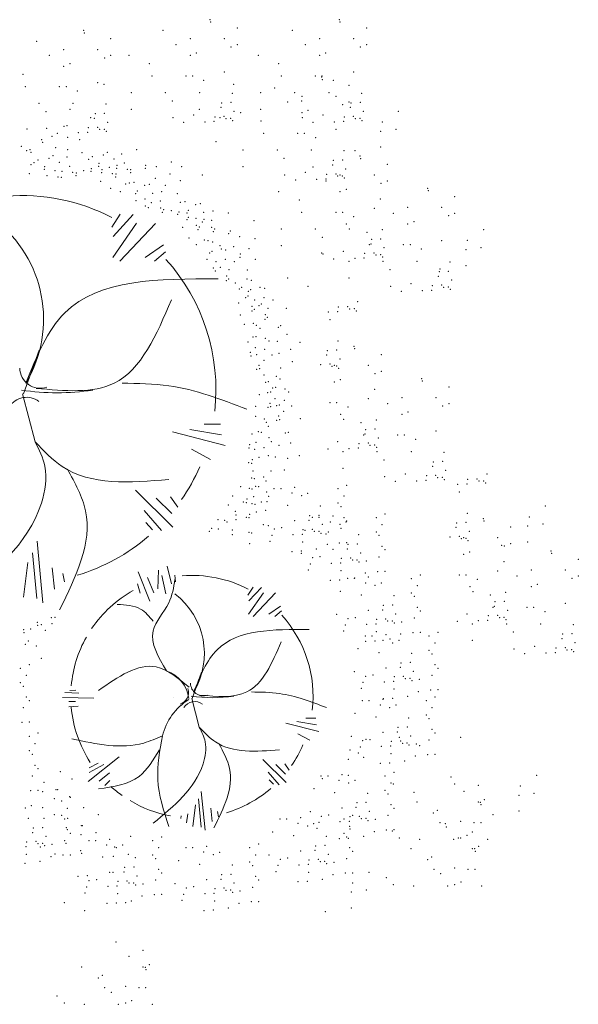
# Model space of a CAD drawing. Units: inches. Extents: x 1239 to 2276906, y 2273 to 321338.
# Tile 21 of 23: x 67989 to 68128, y 11297 to 11541. Entities that reach past the tile are written whole.
import ezdxf

# ---------------------------------------------------------------- set-up
doc = ezdxf.new("R2010")
doc.units = ezdxf.units.IN
doc.layers.add('L-PLNT', color=94, linetype='Continuous', lineweight=13)

# ---------------------------------------------------------------- blocks, each defined once
blk = doc.blocks.new('A$C30B31857')
for p, q in [((3.7503, 4.8792), (3.8028, 4.9604)), ((3.7602, 4.8213), (3.8844, 4.9577)), ((3.7571, 4.688), (3.9054, 4.9034)), ((3.8017, 4.6661), (4.0258, 4.9023)), ((3.9592, 4.6879), (4.0761, 4.7684)), ((4.0192, 4.6658), (4.0886, 4.7234)), ((3.1958, 3.8318), (3.2938, 4.1078)), ((3.1896, 3.8318), (3.2693, 3.5312)), ((4.4619, 3.5087), (4.1316, 3.5937)), ((4.4386, 3.5753), (4.2411, 3.6098)), ((4.4331, 3.6423), (4.3299, 3.6433)), ((4.3707, 3.4211), (4.2509, 3.485)), ((4.1343, 2.9958), (3.8994, 3.2279)), ((4.1284, 3.0819), (4.0285, 3.1775)), ((4.1656, 3.1221), (4.1189, 3.1852)), ((4.0628, 2.975), (3.9547, 3.1008)), ((4.0069, 2.9798), (3.9644, 3.0251)), ((3.3185, 2.5196), (3.2812, 2.9071)), ((3.2801, 2.5477), (3.2528, 2.8343)), ((3.196, 2.5571), (3.224, 2.7743)), ((3.39, 2.6068), (3.3766, 2.7403)), ((4.0388, 2.6092), (4.0438, 2.7263)), ((4.1263, 2.6395), (4.0978, 2.7511)), ((3.4532, 2.6516), (3.4426, 2.7052)), ((3.9897, 2.5318), (3.9158, 2.7153)), ((4.0155, 2.5826), (3.975, 2.6798)), ((4.0896, 2.578), (4.065, 2.6912)), ((4.1506, 2.6527), (4.1457, 2.6942)), ((3.928, 2.5823), (3.9112, 2.6389)), ((4.6056, 2.5687), (4.6384, 2.6195)), ((4.6118, 2.5325), (4.6895, 2.6178)), ((4.6098, 2.4492), (4.7026, 2.5839)), ((4.6377, 2.4355), (4.7778, 2.5831)), ((4.7362, 2.4491), (4.8093, 2.4995)), ((4.7737, 2.4353), (4.8171, 2.4714)), ((4.256, 1.9202), (4.3148, 2.0859)), ((3.4418, 1.9254), (3.6381, 1.9223)), ((3.4556, 1.9575), (3.5427, 1.954)), ((3.488, 1.9706), (3.5256, 1.9718)), ((4.2523, 1.9202), (4.3001, 1.7399)), ((3.4801, 1.8674), (3.5393, 1.8722)), ((3.4804, 1.9008), (3.5234, 1.9004)), ((5.0324, 1.7957), (4.9679, 1.7963)), ((5.0504, 1.7122), (4.8439, 1.7653)), ((5.0358, 1.7538), (4.9124, 1.7754)), ((4.9934, 1.6574), (4.9185, 1.6973)), ((3.6033, 1.3996), (3.7969, 1.5536)), ((3.608, 1.4856), (3.6648, 1.5146)), ((3.6093, 1.4548), (3.7012, 1.505)), ((4.8456, 1.3916), (4.6988, 1.5367)), ((4.8419, 1.4454), (4.7795, 1.5052)), ((4.8652, 1.4705), (4.836, 1.51)), ((3.6717, 1.4005), (3.7356, 1.4536)), ((4.8009, 1.3786), (4.7333, 1.4572)), ((3.7064, 1.3744), (3.739, 1.4052)), ((4.766, 1.3816), (4.7394, 1.4099)), ((4.3358, 1.094), (4.3124, 1.3362)), ((4.2592, 1.1174), (4.2766, 1.2532)), ((4.3117, 1.1115), (4.2947, 1.2906)), ((4.1844, 1.1665), (4.1872, 1.1826)), ((4.2206, 1.1393), (4.2277, 1.1957)), ((4.3805, 1.1485), (4.3721, 1.2319)), ((4.4199, 1.1765), (4.4133, 1.21))]:
    blk.add_line(p, q)
for centre, radius, start, end in [((3.1873, 3.861), 1.217, 62.40199, 94.67087), ((2.5377, 4.3028), 0.7844, 329.07822, 52.6009), ((3.1873, 3.861), 1.217, 353.50541, 42.09121), ((3.3005, 3.9951), 0.1272, 180.26687, 289.21544), ((3.4071, 5.3392), 1.4997, 261.42775, 278.57225), ((3.2157, 3.6838), 0.1272, 52.7337, 148.31892), ((3.1873, 3.861), 1.217, 325.31812, 336.41917), ((3.1873, 3.861), 1.217, 286.50052, 310.70203), ((4.2538, 1.9324), 0.7606, 62.40199, 94.67087), ((4.2538, 1.9324), 0.7606, 118.93501, 145.86797), ((3.8611, 2.2029), 0.4706, 329.07822, 52.6009), ((4.2538, 1.9324), 0.7606, 353.50541, 42.09121), ((4.2538, 1.9324), 0.7606, 150.59537, 174.9599), ((4.0258, 1.8951), 0.2096, 6.88406, 70.93506), ((4.153, 1.9587), 0.0795, 289.21544, 17.13172), ((4.3245, 2.0162), 0.0795, 180.26687, 289.21544), ((4.2203, 1.9258), 0.0795, 179.43656, 180.26687), ((4.3827, 2.8247), 0.8998, 261.42775, 278.57225), ((4.2538, 1.9324), 0.7606, 185.11549, 212.96103), ((4.4263, 1.5995), 0.3678, 121.54331, 166.60172), ((4.2715, 1.8216), 0.0795, 52.7337, 148.31892), ((4.2538, 1.9324), 0.7606, 325.31812, 336.41917), ((4.2538, 1.9324), 0.7606, 227.99389, 234.92066), ((4.2538, 1.9324), 0.7606, 286.50052, 310.70203), ((4.2538, 1.9324), 0.7606, 239.25491, 259.86097)]:
    blk.add_arc(centre, radius, start, end)
for points, knots in [([(3.2106, 3.8997), (3.2782, 4.0657), (3.478, 4.5561), (4.0445, 4.5549), (4.4191, 4.5541)], [0, 0, 0, 0, 0.505063, 1.491803, 1.491803, 1.491803, 1.491803]), ([(3.2759, 3.867), (3.4546, 3.8509), (3.8645, 3.8139), (4.0311, 4.2035), (4.1251, 4.4232)], [0, 0, 0, 0, 0.49103, 1.125938, 1.125938, 1.125938, 1.125938]), ([(3.8148, 3.8997), (3.9136, 3.8984), (4.1838, 3.8949), (4.4376, 3.7978), (4.5987, 3.7361)], [0, 0, 0, 0, 0.29442, 0.8060024, 0.8060024, 0.8060024, 0.8060024]), ([(3.2693, 3.5312), (3.2945, 3.4812), (3.355, 3.361), (3.2868, 2.9371), (3.0051, 2.7057), (2.786, 2.5256)], [0, 0, 0, 0, 0.165135, 0.396758, 1.208872, 1.208872, 1.208872, 1.208872]), ([(3.2693, 3.5312), (3.3234, 3.4742), (3.5366, 3.2499), (3.8644, 3.2754), (4.1088, 3.2945)], [0, 0, 0, 0, 0.229976, 0.9045396, 0.9045396, 0.9045396, 0.9045396]), ([(3.4719, 3.3599), (3.5196, 3.2734), (3.6746, 2.9922), (3.5259, 2.6875), (3.4229, 2.4766)], [0, 0, 0, 0, 0.2856103, 0.9283265, 0.9283265, 0.9283265, 0.9283265]), ([(4.0943, 2.0932), (4.0431, 2.1794), (3.9528, 2.3314), (4.1194, 2.5003), (4.1389, 2.6174), (4.1473, 2.6677)], [0, 0, 0, 0, 0.2643394, 0.4663641, 0.6187177, 0.6187177, 0.6187177, 0.6187177]), ([(4.0102, 2.4054), (3.986, 2.4345), (3.9287, 2.5035), (3.8375, 2.508), (3.7847, 2.5106)], [0, 0, 0, 0, 0.1091589, 0.2590609, 0.2590609, 0.2590609, 0.2590609]), ([(4.2649, 1.961), (4.3054, 2.0606), (4.4253, 2.3548), (4.7652, 2.3541), (4.99, 2.3536)], [0, 0, 0, 0, 0.303038, 0.8950819, 0.8950819, 0.8950819, 0.8950819]), ([(4.3041, 1.9414), (4.4113, 1.9317), (4.6572, 1.9095), (4.7572, 2.1433), (4.8136, 2.2751)], [0, 0, 0, 0, 0.2946182, 0.675563, 0.675563, 0.675563, 0.675563]), ([(4.2355, 1.9904), (4.1681, 2.0469), (3.9917, 2.1946), (3.7911, 2.0563), (3.6671, 1.9708)], [0, 0, 0, 0, 0.2421239, 0.6334325, 0.6334325, 0.6334325, 0.6334325]), ([(4.6274, 1.961), (4.6866, 1.9602), (4.8488, 1.9581), (5.0011, 1.8998), (5.0978, 1.8629)], [0, 0, 0, 0, 0.176652, 0.4836014, 0.4836014, 0.4836014, 0.4836014]), ([(4.3001, 1.7399), (4.3152, 1.7099), (4.3515, 1.6377), (4.3106, 1.3834), (4.1416, 1.2446), (4.0101, 1.1365)], [0, 0, 0, 0, 0.0990809, 0.2380551, 0.7253232, 0.7253232, 0.7253232, 0.7253232]), ([(4.3001, 1.7399), (4.3326, 1.7057), (4.4604, 1.5711), (4.6571, 1.5864), (4.8038, 1.5978)], [0, 0, 0, 0, 0.1379856, 0.5427238, 0.5427238, 0.5427238, 0.5427238]), ([(4.0689, 1.6862), (4.0299, 1.669), (3.8517, 1.5906), (3.6546, 1.6333), (3.5005, 1.6666)], [0, 0, 0, 0, 0.1264411, 0.5776247, 0.5776247, 0.5776247, 0.5776247]), ([(4.0689, 1.6862), (4.0518, 1.5941), (4.0159, 1.4014), (4.0764, 1.2145), (4.1081, 1.1169)], [0, 0, 0, 0, 0.2763889, 0.5787232, 0.5787232, 0.5787232, 0.5787232]), ([(4.4216, 1.6371), (4.4503, 1.5852), (4.5433, 1.4165), (4.454, 1.2337), (4.3922, 1.1071)], [0, 0, 0, 0, 0.1713662, 0.5569959, 0.5569959, 0.5569959, 0.5569959]), ([(4.0493, 1.5978), (4.0122, 1.5345), (3.928, 1.3908), (3.7607, 1.3662), (3.6671, 1.3525)], [0, 0, 0, 0, 0.2099222, 0.4765171, 0.4765171, 0.4765171, 0.4765171])]:
    blk.add_open_spline(points, degree=3, knots=knots)
for p in [(4.3671, 6.1817), (5.1793, 6.1817), (4.3711, 6.1664), (4.5382, 6.1295), (5.1833, 6.1664), (5.3504, 6.1295), (3.5734, 6.1141), (3.5774, 6.0988), (3.7445, 6.0619), (4.0717, 6.1142), (4.2428, 6.062), (4.4567, 6.062), (4.8839, 6.1142), (5.055, 6.062), (5.2689, 6.062), (3.278, 6.0466), (4.1532, 6.025), (4.4994, 6.0098), (4.5382, 6.025), (4.9654, 6.025), (5.3116, 6.0098), (5.3504, 6.025), (3.3595, 5.9574), (3.4491, 5.9944), (3.6629, 5.9944), (3.7057, 5.9422), (3.7445, 5.9574), (3.8578, 5.9575), (4.2428, 5.9575), (4.2816, 5.9728), (4.67, 5.9575), (5.055, 5.9575), (5.0937, 5.9728), (3.4491, 5.8899), (3.4878, 5.9052), (3.9861, 5.9053), (4.7983, 5.9053), (3.1924, 5.8377), (4.002, 5.8283), (4.2159, 5.8283), (4.2586, 5.8283), (4.4567, 5.8531), (4.8142, 5.8283), (5.0281, 5.8283), (5.0685, 5.8211), (5.0708, 5.8283), (5.2689, 5.8531), (3.2083, 5.7607), (3.4221, 5.7607), (3.4649, 5.7607), (3.6629, 5.7855), (3.7026, 5.7761), (4.3283, 5.8008), (4.5148, 5.7761), (4.7731, 5.7537), (5.0726, 5.8059), (5.1405, 5.8008), (5.2396, 5.7689), (3.5346, 5.7332), (3.8737, 5.7238), (4.0876, 5.7238), (4.3014, 5.7238), (4.507, 5.7196), (4.6859, 5.7238), (4.8997, 5.7238), (4.9442, 5.7014), (5.1136, 5.7238), (5.1581, 5.7014), (5.3192, 5.7196), (3.2938, 5.6562), (3.5077, 5.6562), (3.7133, 5.652), (4.1303, 5.6716), (4.4356, 5.6305), (4.44, 5.6593), (4.4982, 5.662), (4.8547, 5.6645), (4.9425, 5.6716), (5.2009, 5.6492), (5.2396, 5.6645), (5.2478, 5.6305), (5.2522, 5.6593), (5.3104, 5.662), (3.3366, 5.604), (3.4887, 5.6194), (3.617, 5.5672), (3.6463, 5.5917), (3.7045, 5.5944), (3.8737, 5.6194), (4.1351, 5.5664), (4.2638, 5.5831), (4.3009, 5.6194), (4.3977, 5.5715), (4.4292, 5.5672), (4.4559, 5.5742), (4.5185, 5.6058), (4.5593, 5.597), (4.6859, 5.6194), (4.9442, 5.597), (4.9473, 5.5664), (4.983, 5.6122), (5.076, 5.5831), (5.2099, 5.5715), (5.2681, 5.5742), (5.3307, 5.6058), (5.5495, 5.607), (3.4498, 5.5125), (3.4701, 5.5155), (3.604, 5.5039), (3.6419, 5.5629), (3.6622, 5.5066), (3.7248, 5.5382), (4.2026, 5.5364), (4.3351, 5.54), (4.3933, 5.5427), (4.4683, 5.5605), (4.4974, 5.5619), (4.5097, 5.5482), (4.6876, 5.5447), (5.0148, 5.5364), (5.1473, 5.54), (5.2055, 5.5427), (5.2804, 5.5605), (5.3095, 5.5619), (5.3219, 5.5482), (5.4484, 5.5393), (3.2183, 5.4955), (3.3414, 5.4988), (3.3754, 5.4495), (3.4088, 5.4688), (3.4726, 5.4423), (3.5414, 5.4724), (3.5996, 5.4751), (3.6745, 5.4929), (3.7036, 5.4943), (3.716, 5.4806), (4.7034, 5.4677), (4.9173, 5.4677), (4.9601, 5.4677), (5.0298, 5.4403), (5.1581, 5.4925), (5.4396, 5.4817), (5.5341, 5.4943), (3.1825, 5.3868), (3.3111, 5.4286), (3.3168, 5.4111), (3.3983, 5.3793), (3.5483, 5.4281), (4.404, 5.4155), (5.4388, 5.3816), (3.2153, 5.3587), (3.2368, 5.3657), (3.2368, 5.3657), (3.2425, 5.3481), (3.3807, 5.3283), (3.4704, 5.3189), (3.474, 5.3651), (3.5639, 5.3462), (3.6293, 5.3208), (3.6985, 5.3321), (3.7228, 5.3481), (3.8125, 5.3386), (3.906, 5.3659), (4.5751, 5.3633), (4.789, 5.3633), (5.0029, 5.3633), (5.2085, 5.359), (5.2765, 5.3597), (5.3085, 5.3254), (3.2439, 5.2709), (3.2628, 5.2851), (3.2872, 5.3011), (3.3282, 5.2596), (3.3564, 5.3123), (3.4217, 5.2869), (3.487, 5.2615), (3.6049, 5.3048), (3.6683, 5.261), (3.6703, 5.2794), (3.7638, 5.3066), (3.7823, 5.2676), (3.8291, 5.2812), (3.9636, 5.2671), (4.0309, 5.26), (4.1244, 5.2873), (4.1902, 5.2588), (4.5751, 5.2588), (4.8318, 5.3111), (5.0131, 5.2579), (5.137, 5.2699), (5.1414, 5.2987), (5.1997, 5.3014), (5.3125, 5.3101), (5.4796, 5.2732), (3.2327, 5.214), (3.3262, 5.2413), (3.3448, 5.2022), (3.3935, 5.2342), (3.4121, 5.1951), (3.4345, 5.1928), (3.4383, 5.2295), (3.5056, 5.2224), (3.5261, 5.2017), (3.528, 5.2201), (3.528, 5.2201), (3.5748, 5.2337), (3.6196, 5.229), (3.6216, 5.2474), (3.6869, 5.2219), (3.6888, 5.2403), (3.7356, 5.2539), (3.7541, 5.2149), (3.7746, 5.1942), (3.7766, 5.2125), (3.7804, 5.2492), (3.8477, 5.2421), (3.8682, 5.2214), (3.8701, 5.2398), (3.8701, 5.2398), (3.9617, 5.2487), (4.1167, 5.2139), (4.3185, 5.2066), (4.8366, 5.2059), (4.9652, 5.2226), (5.0991, 5.2109), (5.1573, 5.2137), (5.1697, 5.2), (5.1842, 5.2057), (5.1988, 5.2013), (5.2199, 5.2452), (5.3981, 5.2057), (3.6811, 5.1669), (3.838, 5.1504), (3.8611, 5.1556), (3.8899, 5.1603), (3.9577, 5.1424), (3.9864, 5.1471), (4.0232, 5.1866), (4.0866, 5.1428), (4.1801, 5.1701), (4.904, 5.1758), (5.0365, 5.1794), (5.0946, 5.1687), (5.0947, 5.1821), (5.2111, 5.1876), (5.4408, 5.1534), (5.4796, 5.1687), (3.7445, 5.1231), (3.8047, 5.1029), (3.9012, 5.0898), (3.9105, 5.1058), (4.007, 5.0926), (4.0645, 5.1021), (4.1611, 5.0889), (4.7992, 5.1012), (5.1842, 5.1012), (5.223, 5.1165), (5.7331, 5.1226), (5.7371, 5.1073), (5.9042, 5.0703), (3.9023, 5.0465), (3.9598, 5.056), (3.9609, 5.0127), (3.9989, 5.0334), (4.0564, 5.0428), (4.1817, 5.0344), (4.2104, 5.0391), (4.2782, 5.0213), (4.3069, 5.026), (4.9275, 5.049), (5.4376, 5.0551), (3.9804, 5.0015), (4.0574, 4.9996), (4.0677, 4.9724), (4.0769, 4.9883), (4.0769, 4.9883), (4.1252, 4.9818), (4.1643, 4.9592), (4.1735, 4.9752), (4.2218, 4.9687), (4.231, 4.9846), (4.3275, 4.9715), (4.385, 4.9809), (4.4816, 4.9678), (4.9434, 4.972), (5.1573, 4.972), (5.2, 4.972), (5.3981, 4.9967), (5.5192, 4.9659), (5.6087, 5.0028), (5.8226, 5.0028), (5.8654, 4.9506), (5.9042, 4.9659), (4.2228, 4.9254), (4.2321, 4.9414), (4.2803, 4.9348), (4.2814, 4.8916), (4.3194, 4.9123), (4.3286, 4.9283), (4.3769, 4.9217), (4.644, 4.9198), (5.2238, 4.8984), (5.2697, 4.9445), (5.6087, 4.8984), (5.6475, 4.9136), (4.1951, 4.8775), (4.2917, 4.8644), (4.3009, 4.8803), (4.3779, 4.8785), (4.3882, 4.8512), (4.3975, 4.8672), (4.3975, 4.8672), (4.4848, 4.8381), (4.494, 4.8541), (4.8151, 4.8675), (5.029, 4.8675), (5.2428, 4.8675), (5.3521, 4.8462), (5.4484, 4.8633), (6.0848, 4.8633), (4.2353, 4.8117), (4.282, 4.7688), (4.3318, 4.7986), (4.355, 4.7939), (4.3832, 4.7865), (4.4301, 4.7631), (4.5526, 4.8203), (4.6491, 4.8072), (4.8151, 4.7631), (5.0717, 4.8153), (5.368, 4.7692), (5.377, 4.7741), (5.3814, 4.8029), (5.4396, 4.8057), (5.5818, 4.7692), (5.6246, 4.7692), (5.8226, 4.7939), (5.9837, 4.7957), (4.3649, 4.7175), (4.3798, 4.7283), (4.4379, 4.7427), (4.4661, 4.7353), (4.5157, 4.7564), (4.5584, 4.7108), (4.6122, 4.7432), (5.0685, 4.7169), (5.0765, 4.7101), (5.2052, 4.7268), (5.3391, 4.7152), (5.3973, 4.7179), (5.4097, 4.7042), (5.4388, 4.7056), (5.4599, 4.7495), (5.6943, 4.7417), (5.9749, 4.7381), (6.0694, 4.7506), (4.3483, 4.6776), (4.4047, 4.6628), (4.4627, 4.6771), (4.5191, 4.6623), (4.5558, 4.6906), (4.6523, 4.6775), (5.144, 4.6801), (5.2396, 4.6647), (5.2765, 4.6836), (5.3347, 4.6864), (5.4511, 4.6919), (5.4535, 4.6647), (5.6674, 4.6647), (5.873, 4.6605), (5.9741, 4.638), (4.388, 4.6229), (4.4013, 4.6046), (4.4312, 4.6263), (4.4875, 4.6115), (4.6019, 4.6111), (5.4963, 4.6125), (5.806, 4.6001), (5.8118, 4.616), (5.8642, 4.6029), (4.4692, 4.5425), (4.4709, 4.5716), (4.4842, 4.5534), (4.4842, 4.5534), (4.5256, 4.5277), (4.5986, 4.5529), (4.6267, 4.5455), (4.8547, 4.5603), (5.2396, 4.5603), (5.6298, 4.524), (5.8016, 4.5713), (5.8219, 4.5151), (5.8845, 4.5466), (4.5521, 4.4913), (4.567, 4.5021), (4.6085, 4.4765), (4.6234, 4.4873), (4.6814, 4.5016), (4.7096, 4.4942), (4.983, 4.508), (5.5011, 4.5073), (5.5685, 4.4772), (5.701, 4.4808), (5.7593, 4.4836), (5.7637, 4.5124), (5.8342, 4.5014), (5.8633, 4.5028), (5.8757, 4.489), (4.547, 4.404), (4.5918, 4.4366), (4.6068, 4.4474), (4.6482, 4.4218), (4.6896, 4.3961), (4.7062, 4.4361), (4.7626, 4.4213), (5.2938, 4.4114), (4.5569, 4.3276), (4.6299, 4.3528), (4.6316, 4.3818), (4.6448, 4.3636), (4.6747, 4.3853), (4.7145, 4.3306), (4.7311, 4.3705), (4.8455, 4.37), (5.1104, 4.3456), (5.1686, 4.3484), (5.173, 4.3772), (5.2312, 4.3799), (5.2435, 4.3662), (5.2726, 4.3675), (5.285, 4.3538), (4.5822, 4.2693), (4.6398, 4.2763), (4.7128, 4.3015), (4.7277, 4.3123), (4.7277, 4.3123), (5.1212, 4.2982), (4.6591, 4.2626), (4.6818, 4.2444), (4.7956, 4.2502), (4.8106, 4.2611), (4.8503, 4.2064), (4.6056, 4.1591), (4.6371, 4.1888), (4.6551, 4.1927), (4.714, 4.1821), (4.7367, 4.1639), (4.7906, 4.163), (4.9332, 4.1551), (5.1715, 4.1647), (4.6197, 4.0929), (4.6511, 4.1227), (4.71, 4.1121), (4.8005, 4.0866), (4.8735, 4.1117), (5.1045, 4.1044), (5.1627, 4.1071), (5.2716, 4.131), (5.2756, 4.1158), (4.6244, 4.0709), (4.6605, 4.0786), (4.706, 4.0421), (4.7554, 4.0757), (4.8833, 4.0353), (5.1001, 4.0756), (5.1204, 4.0193), (5.183, 4.0509), (5.4427, 4.0788), (4.6612, 3.9865), (4.6746, 4.0124), (4.6792, 3.9904), (4.6792, 3.9904), (4.8103, 3.9952), (5.0622, 4.0166), (5.1328, 4.0056), (5.1473, 4.0113), (5.1619, 4.007), (5.1742, 3.9933), (5.3611, 4.0113), (5.4039, 3.9591), (5.4427, 3.9743), (4.7067, 3.9501), (4.716, 3.906), (4.7341, 3.9098), (4.7836, 3.9434), (4.8063, 3.9252), (5.1473, 3.9069), (5.186, 3.9221), (5.6961, 3.9282), (5.7001, 3.913), (4.7301, 3.8399), (4.7482, 3.8437), (4.7615, 3.8696), (4.7796, 3.8734), (4.8384, 3.8629), (4.8612, 3.8447), (5.4007, 3.8607), (5.8672, 3.876), (4.6759, 3.8283), (4.7442, 3.7737), (4.7756, 3.8034), (4.8344, 3.7929), (5.1204, 3.7776), (5.1631, 3.7776), (5.3611, 3.8024), (5.4823, 3.7715), (5.5718, 3.8085), (5.7857, 3.8085), (5.8672, 3.7715), (4.6539, 3.7545), (4.7308, 3.7478), (4.7489, 3.7517), (4.785, 3.7593), (4.803, 3.7632), (4.8304, 3.7229), (4.8799, 3.7565), (5.2328, 3.7502), (5.6106, 3.7193), (5.8285, 3.7563), (4.6533, 3.691), (4.7088, 3.674), (4.7208, 3.6536), (4.7857, 3.6673), (4.799, 3.6932), (4.8037, 3.6711), (4.8037, 3.6711), (4.9348, 3.6759), (5.1869, 3.704), (5.2059, 3.6732), (5.3152, 3.6518), (5.4115, 3.6689), (5.5718, 3.704), (4.6707, 3.5951), (4.6887, 3.5913), (4.7342, 3.6277), (4.8405, 3.5868), (4.8586, 3.5906), (5.3445, 3.6086), (5.4027, 3.6113), (5.7857, 3.5996), (4.6299, 3.5808), (4.6566, 3.529), (4.7382, 3.5578), (4.7515, 3.5319), (4.8726, 3.5245), (5.1683, 3.5325), (5.331, 3.5748), (5.3401, 3.5798), (5.423, 3.5551), (5.5449, 3.5748), (5.5877, 3.5748), (5.6574, 3.5474), (4.6111, 3.4926), (4.6158, 3.5146), (4.6472, 3.4849), (4.7061, 3.4954), (4.8004, 3.5091), (5.1071, 3.4857), (5.2027, 3.4704), (5.2396, 3.4893), (5.2978, 3.492), (5.3022, 3.5208), (5.3604, 3.5236), (5.3727, 3.5099), (5.4018, 3.5112), (5.4142, 3.4975), (5.4166, 3.4704), (5.6305, 3.4704), (5.8361, 3.4661), (4.6104, 3.4005), (4.6332, 3.4187), (4.674, 3.4331), (4.7328, 3.4437), (4.7784, 3.4353), (4.8553, 3.4286), (4.9275, 3.4439), (5.4594, 3.4181), (5.769, 3.4058), (5.8273, 3.4085), (4.6285, 3.3967), (4.6285, 3.3967), (4.6372, 3.3488), (4.7502, 3.3478), (4.8332, 3.3548), (5.2027, 3.3659), (5.7646, 3.377), (5.8475, 3.3523), (4.6278, 3.3047), (4.6458, 3.3008), (4.7047, 3.3114), (4.718, 3.2855), (5.4642, 3.3129), (5.5316, 3.2829), (5.5928, 3.3297), (5.6641, 3.2865), (5.7223, 3.2892), (5.7267, 3.318), (5.7849, 3.3208), (5.7973, 3.307), (5.8264, 3.3084), (5.8387, 3.2947), (5.9852, 3.2955), (6.0434, 3.2982), (6.0557, 3.2845), (6.0848, 3.2859), (6.106, 3.3298), (4.5596, 3.25), (4.6137, 3.2385), (4.6318, 3.2347), (4.6545, 3.2529), (4.6726, 3.2491), (4.722, 3.2155), (4.7696, 3.2368), (4.8124, 3.2368), (4.8997, 3.2451), (5.1707, 3.2366), (5.2261, 3.2591), (5.9226, 3.2639), (5.9334, 3.2165), (5.9808, 3.2667), (6.0972, 3.2722), (4.5094, 3.1915), (4.5769, 3.1541), (4.5997, 3.1724), (4.6404, 3.1867), (4.6899, 3.1532), (4.7246, 3.1559), (4.7354, 3.1896), (4.8821, 3.2093), (4.9424, 3.1929), (4.9812, 3.2082), (5.2076, 3.1915), (4.483, 3.1338), (4.5268, 3.0957), (4.595, 3.1503), (4.6311, 3.1426), (4.6491, 3.1388), (4.6578, 3.0909), (4.7167, 3.1014), (4.8552, 3.1323), (5.0608, 3.1281), (5.1707, 3.1464), (5.1892, 3.1239), (6.4724, 3.1281), (4.4168, 3.0426), (4.4599, 3.0391), (4.5295, 3.0722), (4.5312, 3.0431), (4.5943, 3.0583), (4.6123, 3.0544), (4.6123, 3.0544), (4.617, 3.0765), (4.8997, 3.0362), (4.9894, 3.039), (4.9938, 3.0678), (5.0096, 3.0565), (5.052, 3.0705), (5.0524, 3.0565), (5.1221, 3.0291), (5.1396, 3.0649), (5.2076, 3.0562), (5.2261, 3.0337), (5.4107, 3.0563), (5.4661, 3.0788), (5.9837, 3.083), (6.0838, 3.0494), (6.0878, 3.0341), (6.3714, 3.0605), (4.3638, 2.9696), (4.377, 2.9879), (4.4201, 2.9844), (4.4748, 3.0283), (4.5064, 2.9775), (4.7017, 3.0115), (4.734, 3.0055), (4.7714, 2.984), (4.8176, 2.9916), (4.9515, 2.98), (4.9645, 2.9757), (5.0097, 2.9827), (5.022, 2.969), (5.0511, 2.9704), (5.0723, 3.0143), (5.1824, 3.0126), (5.1892, 2.9886), (5.2212, 3.0279), (5.4476, 3.0112), (5.9123, 2.9939), (5.9167, 3.0227), (5.9749, 3.0254), (5.9952, 2.9692), (6.2549, 2.9971), (6.3626, 3.0029), (6.4571, 3.0154), (4.508, 2.9484), (4.6116, 2.9624), (4.6297, 2.9586), (4.7444, 2.907), (4.7563, 2.9449), (4.8889, 2.9485), (4.9471, 2.9512), (5.0635, 2.9567), (5.0952, 2.9521), (5.1094, 2.9645), (5.3008, 2.9478), (5.4107, 2.9661), (5.4292, 2.9436), (5.8744, 2.9349), (5.9326, 2.9377), (5.945, 2.9239), (5.9595, 2.9296), (5.9741, 2.9253), (5.9864, 2.9116), (6.1733, 2.9296), (4.6156, 2.8924), (4.9412, 2.8452), (4.95, 2.9027), (5.0357, 2.8577), (5.1032, 2.8877), (5.1396, 2.8559), (5.1798, 2.8972), (5.2261, 2.8984), (5.2293, 2.8587), (5.2337, 2.8875), (5.2919, 2.8902), (5.4476, 2.8759), (5.4661, 2.8534), (6.1994, 2.8809), (6.2161, 2.8774), (6.2549, 2.8927), (6.3617, 2.9028), (6.5083, 2.8465), (4.883, 2.8424), (4.9416, 2.8312), (5.0113, 2.8037), (5.0575, 2.8114), (5.1914, 2.7997), (5.2496, 2.8025), (5.262, 2.7887), (5.2911, 2.7901), (5.3122, 2.834), (5.3494, 2.7842), (5.4292, 2.8083), (5.9595, 2.8252), (5.9982, 2.8404), (6.5123, 2.8313), (6.6794, 2.7943), (4.9844, 2.7267), (4.9963, 2.7646), (5.1288, 2.7682), (5.187, 2.7709), (5.19, 2.7225), (5.3034, 2.7764), (6.1733, 2.7207), (6.2129, 2.7791), (6.384, 2.7268), (6.5979, 2.7268), (5.123, 2.6621), (5.1812, 2.6649), (5.2311, 2.6734), (5.2739, 2.6734), (5.2757, 2.6774), (5.3431, 2.7074), (5.3611, 2.6818), (5.4198, 2.7169), (5.4661, 2.7181), (5.6322, 2.6732), (5.6876, 2.6957), (5.9325, 2.696), (5.9753, 2.696), (6.045, 2.6685), (6.2945, 2.6899), (6.6407, 2.6746), (6.6794, 2.6899), (5.3436, 2.646), (5.4039, 2.6295), (5.4427, 2.6448), (5.6691, 2.6281), (5.999, 2.6224), (6.384, 2.6224), (6.4228, 2.6376), (5.186, 2.5926), (5.3167, 2.569), (5.5223, 2.5647), (5.6322, 2.583), (5.6507, 2.5605), (6.0181, 2.5915), (6.1274, 2.5701), (6.2237, 2.5873), (5.3611, 2.4728), (5.4508, 2.4756), (5.4552, 2.5044), (5.5135, 2.5071), (5.6691, 2.4929), (6.1432, 2.4932), (6.1523, 2.4981), (6.1567, 2.5269), (6.2149, 2.5297), (6.2352, 2.4734), (6.3571, 2.4932), (6.3999, 2.4932), (6.5979, 2.5179), (3.371, 2.4265), (3.3934, 2.4288), (5.1631, 2.4481), (5.2328, 2.4206), (5.279, 2.4283), (5.4129, 2.4166), (5.4711, 2.4194), (5.5337, 2.4509), (5.6507, 2.4252), (5.6876, 2.4703), (5.9805, 2.4508), (6.1144, 2.4392), (6.1726, 2.4419), (6.1849, 2.4282), (6.214, 2.4296), (6.2264, 2.4158), (6.4696, 2.4657), (3.1974, 2.3525), (3.2423, 2.3573), (3.2832, 2.3987), (3.2852, 2.3803), (3.2852, 2.3803), (3.3076, 2.3827), (3.3748, 2.3897), (5.2178, 2.3815), (5.3503, 2.3851), (5.4085, 2.3878), (5.4835, 2.4056), (5.5126, 2.407), (5.5249, 2.3933), (5.5709, 2.4011), (5.9192, 2.404), (6.0149, 2.3887), (6.0518, 2.4076), (6.11, 2.4104), (6.2288, 2.3887), (6.4426, 2.3887), (6.6482, 2.3844), (3.1994, 2.3342), (3.3339, 2.3483), (5.2059, 2.3436), (5.3419, 2.3129), (5.3846, 2.3129), (5.4115, 2.3394), (5.4719, 2.3212), (5.4972, 2.2943), (5.5646, 2.3243), (5.6413, 2.3338), (5.6876, 2.3351), (5.743, 2.3126), (5.7983, 2.3352), (6.2715, 2.3365), (6.5768, 2.2953), (6.5812, 2.3241), (6.6394, 2.3268), (3.2071, 2.2608), (3.2276, 2.2815), (3.2763, 2.2495), (5.2968, 2.232), (5.3445, 2.279), (5.4027, 2.2818), (5.4543, 2.2854), (5.5147, 2.269), (5.5534, 2.2842), (5.7799, 2.2676), (6.0149, 2.2842), (6.2764, 2.2313), (6.405, 2.248), (6.5389, 2.2363), (6.5971, 2.2391), (6.6386, 2.2267), (6.6597, 2.2706), (3.3085, 2.1726), (5.4274, 2.2084), (5.633, 2.2042), (5.743, 2.2225), (5.7614, 2.1999), (6.3438, 2.2012), (6.4763, 2.2048), (6.5345, 2.2075), (6.6095, 2.2254), (6.6509, 2.213), (3.1772, 2.1098), (3.2325, 2.1324), (5.4719, 2.1123), (5.5616, 2.115), (5.566, 2.1438), (5.6242, 2.1466), (5.7799, 2.1323), (5.7983, 2.1098), (3.2141, 2.0647), (5.2739, 2.0875), (5.3436, 2.0601), (5.3898, 2.0677), (5.5237, 2.0561), (5.5819, 2.0588), (5.5942, 2.0451), (5.6233, 2.0465), (5.6445, 2.0903), (5.6816, 2.0406), (5.7614, 2.0647), (3.1772, 2.0197), (3.1956, 1.9971), (5.3167, 1.9831), (5.3286, 2.0209), (5.4611, 2.0245), (5.5193, 2.0273), (5.5223, 1.9788), (5.6357, 2.0327), (3.2141, 1.9295), (5.4552, 1.9185), (5.5135, 1.9212), (5.608, 1.9338), (5.6754, 1.9638), (5.752, 1.9732), (5.7799, 1.9296), (5.7983, 1.9745), (3.1956, 1.8619), (3.2325, 1.9069), (5.3234, 1.9072), (5.3662, 1.9072), (5.4359, 1.8798), (5.4534, 1.9156), (5.4962, 1.8633), (5.535, 1.8786), (5.7245, 1.907), (5.7614, 1.8619), (5.2783, 1.8264), (5.409, 1.8028), (5.6146, 1.7985), (5.7245, 1.8168), (5.743, 1.7943), (3.1862, 1.7704), (3.2325, 1.7717), (5.5475, 1.7382), (5.6057, 1.7409), (3.2326, 1.6817), (3.2879, 1.7042), (5.2554, 1.6819), (5.4534, 1.7067), (5.5431, 1.7094), (5.5561, 1.6758), (5.626, 1.6847), (5.7614, 1.7267), (5.7799, 1.7041), (5.9411, 1.6758), (3.2695, 1.6366), (5.3101, 1.6153), (5.3251, 1.6544), (5.3465, 1.6634), (5.3713, 1.6621), (5.4426, 1.6189), (5.5008, 1.6216), (5.5052, 1.6504), (5.5634, 1.6532), (5.5758, 1.6395), (5.6049, 1.6408), (5.6172, 1.6271), (5.6632, 1.635), (5.6844, 1.6236), (5.743, 1.659), (3.2326, 1.5915), (3.251, 1.569), (5.2454, 1.5957), (5.2982, 1.5774), (5.3311, 1.5507), (5.5038, 1.5732), (5.6569, 1.5582), (5.7336, 1.5676), (5.7799, 1.5689), (3.2695, 1.5013), (5.2366, 1.5381), (5.4368, 1.5129), (5.495, 1.5156), (5.5895, 1.5281), (3.251, 1.4337), (3.2879, 1.4788), (3.4267, 1.4606), (5.065, 1.434), (5.1078, 1.434), (5.195, 1.4423), (5.2357, 1.438), (5.4661, 1.4338), (5.5214, 1.4563), (5.8807, 1.427), (6.4171, 1.438), (3.3257, 1.3929), (3.5006, 1.4155), (5.0734, 1.4161), (5.1774, 1.4065), (5.2378, 1.3901), (5.2766, 1.4054), (5.503, 1.3887), (5.5192, 1.3828), (5.9042, 1.3828), (6.0518, 1.3747), (6.316, 1.3704), (3.2416, 1.3422), (3.2879, 1.3435), (3.3169, 1.3353), (3.3995, 1.3478), (3.4114, 1.3479), (3.4852, 1.3028), (3.491, 1.2986), (5.0199, 1.3531), (5.1505, 1.3296), (5.3561, 1.3253), (5.4661, 1.3436), (5.4845, 1.3211), (5.6475, 1.3306), (5.9622, 1.3378), (6.3072, 1.3128), (6.4017, 1.3253), (3.2461, 1.2476), (3.3907, 1.2902), (3.4356, 1.276), (5.2891, 1.265), (5.3473, 1.2677), (5.503, 1.2534), (5.6668, 1.2703), (6.0518, 1.2703), (6.0653, 1.2691), (6.0693, 1.2539), (6.0905, 1.2855), (3.2073, 1.2324), (3.316, 1.2352), (3.3898, 1.1901), (3.4356, 1.1859), (3.4725, 1.231), (3.5744, 1.2352), (3.6667, 1.1901), (4.997, 1.2087), (5.0667, 1.1812), (5.1129, 1.1889), (5.195, 1.2334), (5.2468, 1.1772), (5.263, 1.1859), (5.2847, 1.2362), (5.305, 1.1799), (5.3676, 1.2115), (5.4845, 1.1858), (5.5214, 1.2309), (5.7699, 1.2016), (5.7951, 1.2181), (6.1441, 1.1907), (6.3063, 1.2127), (3.2276, 1.1682), (3.3257, 1.1676), (3.4541, 1.1633), (3.4733, 1.1676), (3.559, 1.1225), (3.5656, 1.1225), (4.8066, 1.1636), (4.8493, 1.1636), (4.919, 1.1361), (4.9366, 1.1719), (4.9794, 1.1197), (5.0181, 1.135), (5.0517, 1.1421), (5.1842, 1.1457), (5.2077, 1.1634), (5.2424, 1.1484), (5.2446, 1.1183), (5.3174, 1.1662), (5.3465, 1.1676), (5.3588, 1.1539), (5.4047, 1.1617), (5.811, 1.1411), (5.8437, 1.134), (5.941, 1.1494), (6.0248, 1.1411), (6.0676, 1.1411), (3.2542, 1.0784), (3.2586, 1.1072), (3.3169, 1.11), (3.3371, 1.0537), (3.4645, 1.11), (3.4725, 1.0957), (3.491, 1.0732), (3.5568, 1.0649), (3.6513, 1.0774), (3.8698, 1.0549), (4.7615, 1.0827), (4.8921, 1.0591), (5.0398, 1.1042), (5.0977, 1.0549), (5.2077, 1.0732), (5.2454, 1.1), (5.3311, 1.0549), (5.3985, 1.0849), (5.4751, 1.0944), (5.5115, 1.0888), (5.5214, 1.0956), (5.8514, 1.1124), (5.9798, 1.0602), (6.0148, 1.0818), (3.2119, 0.9907), (3.2163, 1.0195), (3.2745, 1.0222), (3.2869, 1.0085), (3.316, 1.0099), (3.3283, 0.9961), (3.3743, 1.004), (3.4541, 1.0281), (3.4637, 1.0099), (3.6067, 1.0284), (3.6495, 1.0284), (3.7192, 1.0009), (3.7368, 1.0367), (3.8183, 0.9997), (4.0078, 1.0282), (4.0632, 1.0507), (4.3459, 0.9916), (4.6723, 1.0056), (5.0307, 0.9946), (5.0889, 0.9973), (5.1784, 1.0396), (5.2261, 1.0506), (5.2366, 1.0424), (5.556, 1.0449), (5.6826, 1.0366), (5.8965, 1.0366), (5.9253, 1.0448), (5.941, 1.0449), (6.0536, 0.9926), (6.1104, 1.0366), (3.2149, 0.9422), (3.3014, 0.9879), (3.3937, 0.9429), (3.4447, 0.9366), (3.491, 0.9379), (3.556, 0.9648), (3.5617, 0.9475), (3.7599, 0.9297), (3.7687, 0.9873), (3.7795, 0.9845), (3.8544, 0.9422), (4.0078, 0.938), (4.0447, 0.9831), (4.2159, 0.9833), (4.2586, 0.9833), (4.3283, 0.9559), (4.3887, 0.9394), (4.4274, 0.9547), (4.617, 0.9831), (4.6539, 0.938), (4.7386, 0.9382), (4.9366, 0.963), (5.0263, 0.9658), (5.1092, 0.9411), (5.2446, 0.983), (5.263, 0.9605), (5.6299, 0.9773), (6.0148, 0.9773), (6.0284, 0.9762), (6.0324, 0.9609), (3.2061, 0.8846), (3.3006, 0.8972), (3.368, 0.9272), (3.6923, 0.9239), (3.8979, 0.9197), (4.0263, 0.9154), (4.1708, 0.9024), (4.3014, 0.8789), (4.507, 0.8746), (4.617, 0.8929), (4.6354, 0.8704), (4.7933, 0.8717), (4.8083, 0.9108), (4.8545, 0.9184), (4.9258, 0.8753), (4.984, 0.878), (4.9884, 0.9068), (5.0466, 0.9095), (5.0589, 0.8958), (5.088, 0.8972), (5.1004, 0.8835), (5.1463, 0.8913), (5.2261, 0.9154), (5.733, 0.9087), (5.7582, 0.9251), (3.5967, 0.8076), (3.7368, 0.8278), (3.759, 0.8296), (3.8265, 0.8305), (3.8309, 0.8593), (3.8891, 0.8621), (3.9094, 0.8059), (4.0447, 0.8478), (4.0632, 0.8253), (4.44, 0.8143), (4.4982, 0.817), (4.7814, 0.8338), (4.987, 0.8295), (5.1401, 0.8145), (5.2167, 0.8239), (5.263, 0.8252), (5.3649, 0.8296), (5.774, 0.8481), (5.8145, 0.8195), (5.9041, 0.8564), (5.9879, 0.8481), (6.0307, 0.8481), (3.5388, 0.803), (3.6084, 0.7756), (3.6547, 0.7832), (3.7842, 0.7428), (3.7886, 0.7716), (3.8468, 0.7743), (3.8591, 0.7606), (3.8882, 0.762), (3.9006, 0.7483), (3.9465, 0.7561), (4.0263, 0.7802), (4.1479, 0.758), (4.3459, 0.7827), (4.4356, 0.7855), (4.5185, 0.7608), (4.6539, 0.8027), (4.6723, 0.7802), (4.9199, 0.7692), (4.9781, 0.7719), (5.0727, 0.7845), (5.2638, 0.7619), (5.4746, 0.7959), (5.5191, 0.752), (5.6457, 0.7436), (5.8596, 0.7436), (5.9041, 0.752), (5.9428, 0.7672), (6.0735, 0.7436), (3.5815, 0.6986), (3.5934, 0.7365), (3.726, 0.74), (3.7871, 0.6943), (4.0169, 0.6887), (4.0632, 0.69), (4.2026, 0.6914), (4.2176, 0.7305), (4.2638, 0.7382), (4.3351, 0.695), (4.3933, 0.6977), (4.3977, 0.7265), (4.4559, 0.7293), (4.4683, 0.7155), (4.4974, 0.7169), (4.5097, 0.7032), (4.5556, 0.711), (4.6354, 0.7351), (5.255, 0.7043), (5.3495, 0.7169), (3.4518, 0.6392), (3.7201, 0.634), (3.7783, 0.6367), (3.8368, 0.6392), (3.8728, 0.6493), (3.9403, 0.6793), (4.1907, 0.6535), (4.3963, 0.6493), (4.5494, 0.6342), (4.626, 0.6437), (4.6723, 0.6449), (3.5801, 0.587), (4.3293, 0.5889), (4.3875, 0.5917), (4.482, 0.6042), (5.0919, 0.5823), (5.2542, 0.6042), (3.7764, 0.3904), (3.9475, 0.3381), (3.8579, 0.3012), (3.9862, 0.2489), (3.5625, 0.2337), (3.9475, 0.2337), (3.961, 0.2325), (3.965, 0.2172), (3.6656, 0.165), (3.6908, 0.1815), (3.7067, 0.1045), (3.7471, 0.0758), (3.8367, 0.1128), (3.9205, 0.1045), (3.9633, 0.1045), (3.4072, 0.0522), (3.4517, 0.0083), (3.5783, 0), (3.7922, 0), (3.8367, 0.0083), (3.8755, 0.0236), (4.0061, 0)]:
    blk.add_point(p)
blk = doc.blocks.new('p2')
at = {"xscale": 1000, "yscale": 1000, "zscale": 1000}
blk.add_blockref('A$C30B31857', (-714.2, -1628.3), dxfattribs=at)

msp = doc.modelspace()

# ---------------------------------------------------------------- block references
at = {"layer": 'L-PLNT', "xscale": 0.0393700787401575, "yscale": 0.0393700787401575, "zscale": 0.0393700787401575}
msp.add_blockref('p2', (67892.66, 11361.51), dxfattribs=at)

doc.saveas('drawing.dxf')
